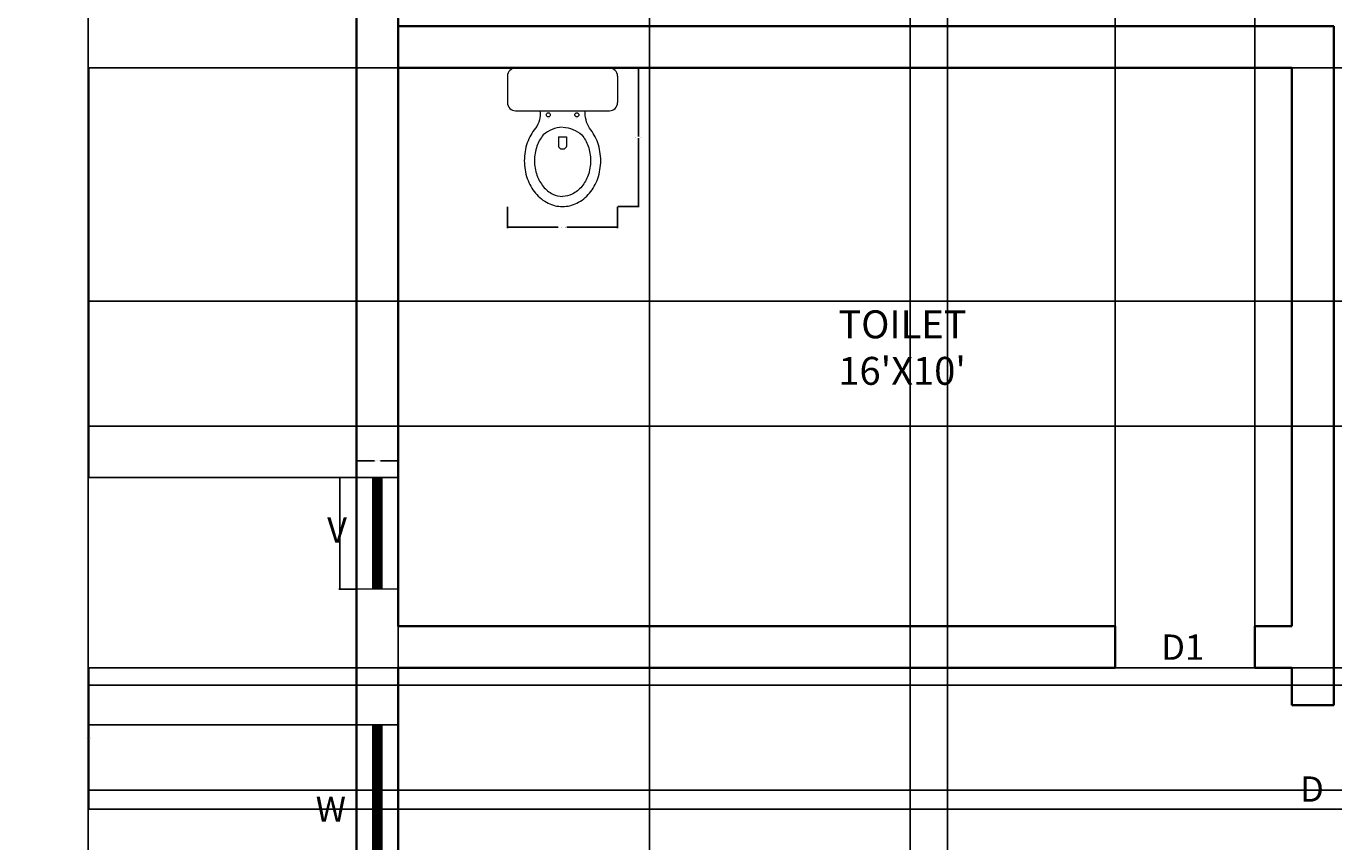
# Model space of a CAD drawing. Units: inches. Extents: x 318 to 927, y -1130 to 13.
# Tile 6 of 17: x 318 to 599, y -867 to -692. Entities that reach past the tile are written whole.
import ezdxf

# ---------------------------------------------------------------- set-up
doc = ezdxf.new("R2010")
doc.units = ezdxf.units.IN
doc.header["$MEASUREMENT"] = 0
for name, color, linetype, lineweight in [('A-ANNO-DIMS', 1, 'Continuous', 18), ('A-ANNO-IDEN', 1, 'Continuous', 13), ('A-AREA-IDEN', 8, 'Continuous', 18), ('A-FLOR-FIXT', 7, 'Continuous', 18), ('A-GLAZ-PATT', 5, 'Continuous', 9), ('wall', 1, 'Continuous', 35), ('win', 5, 'Continuous', 18)]:
    doc.layers.add(name, color=color, linetype=linetype, lineweight=lineweight)
doc.styles.get("Standard").update_dxf_attribs({"font": 'arial.ttf'})
doc.dimstyles.get("Standard").update_dxf_attribs({"dimtxt": 0.18, "dimasz": 0.18, "dimexe": 0.18, "dimexo": 0.0625, "dimgap": 0.09, "dimtad": 0, "dimtih": 1, "dimtoh": 1, "dimdec": 1, "dimzin": 0, "dimdsep": 46, "dimlunit": 4, "dimtxsty": 'Standard', "dimcen": 0.09, "dimadec": 0, "dimazin": 0, "dimtfac": 1, "dimtdec": 1, "dimtofl": 0, "dimtmove": 0, "dimatfit": 3, "dimfxl": 1, "dimtolj": 1, "dimtzin": 0, "dimarcsym": 0})

# ---------------------------------------------------------------- blocks, each defined once
blk = doc.blocks.new('WC-P01')
for p, q in [((-230, 0), (230, 0)), ((-270, -40), (-270, -170)), ((270, -40), (270, -170)), ((-230, -210), (230, -210)), ((-111.4, -210), (-111.4, -210)), ((-20, -337.8), (20, -337.8)), ((-20, -337.8), (-20, -385.7)), ((20, -337.8), (20, -385.7)), ((-18.5, -389.3), (-10.5, -397.3)), ((-10.5, -397.3), (10.5, -397.3)), ((10.5, -397.3), (18.5, -389.3))]:
    blk.add_line(p, q)
for points in [[(-111.4, -210, -0.215497), (-132.6, -295.9, 0.09084), (-172.8, -367.1, 0.083285), (-187.5, -455, 0.083285), (-172.8, -542.9, 0.09084), (-132.6, -614.1, 0.104065), (-70, -663.6, 0.115836), (0, -680, 0.115836), (70, -663.6, 0.104065), (132.6, -614.1, 0.09084), (172.8, -542.9, 0.083285), (187.5, -455, 0.083285)], [(-70, -246.4), (-70, -246.4, 0.104065)], [(70, -246.4), (70, -246.4, 0.115836)], [(187.5, -455, 0.083285), (172.8, -367.1, 0.09084), (132.6, -295.9, -0.156524), (111.4, -210)], [(-1.8, -291.3, 0.171753), (-94.2, -327.9, 0.09084), (-125.5, -383.5, 0.083285), (-137.5, -455, 0.083285), (-125.5, -526.5, 0.09084), (-94.2, -582.1, 0.104065), (-47.7, -618.8, 0.115836), (0, -630, 0.115836)], [(1.8, -291.3, -0.171753), (94.2, -327.9, -0.09084), (125.5, -383.5, -0.083285), (137.5, -455, -0.083285), (125.5, -526.5, -0.09084), (94.2, -582.1, -0.104065), (47.7, -618.8, -0.115836), (0, -630, -0.115836)]]:
    blk.add_lwpolyline(points, format="xyb")
for centre in [(-70, -230), (70, -230)]:
    blk.add_circle(centre, 10)
for centre, radius, start, end in [((-230, -40), 40, 90, 180), ((230, -40), 40, 0, 90), ((-230, -170), 40, 180, 270), ((230, -170), 40, 270, 0), ((-15, -385.7), 5, 180, 225), ((15, -385.7), 5, 315, 0)]:
    blk.add_arc(centre, radius, start, end)
blk = doc.blocks.new('_ArchTick')
at = {"color": 0, "linetype": 'ByBlock', "const_width": 0.15}
blk.add_lwpolyline([(-0.5, -0.5), (0.5, 0.5)], dxfattribs=at)
blk = doc.blocks.new('*D4')
at = {"layer": 'A-ANNO-DIMS', "color": 0, "lineweight": -2, "transparency": 16777216}
blk.add_line((331.26, -82.91), (331.26, -1042.91), dxfattribs=at)
at = {"layer": 'Defpoints', "color": 0, "transparency": 16777216}
for p in [(388.89, -82.91), (331.26, -1042.91), (388.89, -1042.91)]:
    blk.add_point(p, dxfattribs=at)
at = {"layer": 'A-ANNO-DIMS', "color": 0, "lineweight": -2, "transparency": 16777216, "xscale": 6, "yscale": 6, "zscale": 6}
for p, rotation in [((331.26, -82.91), 90), ((331.26, -1042.91), 270)]:
    blk.add_blockref('_ArchTick', p, dxfattribs=dict(at, rotation=rotation))
at = {"layer": 'A-ANNO-DIMS', "color": 0, "transparency": 16777216, "insert": (323.18, -562.91), "char_height": 8, "attachment_point": 5, "rotation": 90}
blk.add_mtext("\\A1;80'", dxfattribs=at)
blk = doc.blocks.new('WIN-36IN')
for p, q in [((0, 36), (9, 36)), ((3.5, 36), (3.5, 0)), ((5.5, 36), (5.5, 0)), ((0, 0), (9, 0))]:
    blk.add_line(p, q)
blk = doc.blocks.new('VENT-24IN')
for p, q in [((9, 24), (0, 24)), ((3.5, 0), (3.5, 24)), ((5.5, 0), (5.5, 24)), ((9, 0), (0, 0))]:
    blk.add_line(p, q)
blk = doc.blocks.new('*D17')
at = {"layer": 'A-ANNO-DIMS', "color": 0, "lineweight": -2, "transparency": 16777216}
for p, q in [((445.06, -700.91), (449.65, -700.91)), ((449.47, -701.09), (449.47, -715.62)), ((449.47, -730.52), (449.47, -715.99)), ((445.06, -730.7), (449.65, -730.7))]:
    blk.add_line(p, q, dxfattribs=at)
at = {"layer": 'A-ANNO-DIMS', "color": 0, "transparency": 16777216}
for points in [[(449.44, -701.09), (449.5, -701.09), (449.47, -700.91)], [(449.44, -730.52), (449.5, -730.52), (449.47, -730.7)]]:
    blk.add_solid(points, dxfattribs=at)
at = {"layer": 'Defpoints', "color": 0, "transparency": 16777216}
for p in [(445, -700.91), (449.47, -700.91), (445, -730.7)]:
    blk.add_point(p, dxfattribs=at)
at = {"layer": 'A-ANNO-DIMS', "color": 0, "transparency": 16777216, "insert": (449.47, -715.81), "char_height": 0.18, "attachment_point": 5}
blk.add_mtext('\\A1;WC 2\'-6" TYP.', dxfattribs=at)
blk = doc.blocks.new('*D18')
at = {"layer": 'A-ANNO-DIMS', "color": 0, "lineweight": -2, "transparency": 16777216}
for p, q in [((421.34, -730.76), (421.34, -735.35)), ((445, -730.76), (445, -735.35)), ((421.52, -735.17), (432.26, -735.17)), ((444.82, -735.17), (434.08, -735.17))]:
    blk.add_line(p, q, dxfattribs=at)
at = {"layer": 'A-ANNO-DIMS', "color": 0, "transparency": 16777216}
for points in [[(421.52, -735.14), (421.52, -735.2), (421.34, -735.17)], [(444.82, -735.14), (444.82, -735.2), (445, -735.17)]]:
    blk.add_solid(points, dxfattribs=at)
at = {"layer": 'Defpoints', "color": 0, "transparency": 16777216}
for p in [(421.34, -730.7), (445, -730.7), (445, -735.17)]:
    blk.add_point(p, dxfattribs=at)
at = {"layer": 'A-ANNO-DIMS', "color": 0, "transparency": 16777216, "insert": (433.17, -735.17), "char_height": 0.18, "attachment_point": 5}
blk.add_mtext('\\A1;1\'-11 1/2" TYP.', dxfattribs=at)
blk = doc.blocks.new('*D21')
at = {"layer": 'A-ANNO-DIMS', "color": 0, "lineweight": -2, "transparency": 16777216}
for p, q in [((388.83, -788.96), (385.11, -788.96)), ((385.29, -789.14), (385.29, -800.78)), ((385.29, -812.78), (385.29, -801.14)), ((388.83, -812.96), (385.11, -812.96))]:
    blk.add_line(p, q, dxfattribs=at)
at = {"layer": 'A-ANNO-DIMS', "color": 0, "transparency": 16777216}
for points in [[(385.26, -789.14), (385.32, -789.14), (385.29, -788.96)], [(385.26, -812.78), (385.32, -812.78), (385.29, -812.96)]]:
    blk.add_solid(points, dxfattribs=at)
at = {"layer": 'Defpoints', "color": 0, "transparency": 16777216}
for p in [(385.29, -788.96), (388.89, -788.96), (388.89, -812.96)]:
    blk.add_point(p, dxfattribs=at)
at = {"layer": 'A-ANNO-DIMS', "color": 0, "transparency": 16777216, "insert": (385.29, -800.96), "char_height": 0.18, "attachment_point": 5}
blk.add_mtext('\\A1;VENT 2\'-0" TYP.', dxfattribs=at)
blk = doc.blocks.new('*D22')
at = {"layer": 'A-ANNO-DIMS', "color": 0, "lineweight": -2, "transparency": 16777216}
for p, q in [((388.89, -788.9), (388.89, -785.18)), ((389.07, -785.36), (392.76, -785.36)), ((397.71, -785.36), (394.03, -785.36)), ((397.89, -788.9), (397.89, -785.18))]:
    blk.add_line(p, q, dxfattribs=at)
at = {"layer": 'A-ANNO-DIMS', "color": 0, "transparency": 16777216}
for points in [[(389.07, -785.33), (389.07, -785.39), (388.89, -785.36)], [(397.71, -785.33), (397.71, -785.39), (397.89, -785.36)]]:
    blk.add_solid(points, dxfattribs=at)
at = {"layer": 'Defpoints', "color": 0, "transparency": 16777216}
for p in [(397.89, -785.36), (388.89, -788.96), (397.89, -788.96)]:
    blk.add_point(p, dxfattribs=at)
at = {"layer": 'A-ANNO-DIMS', "color": 0, "transparency": 16777216, "insert": (393.39, -785.36), "char_height": 0.18, "attachment_point": 5}
blk.add_mtext('\\A1;0\'-9" TYP.', dxfattribs=at)
blk = doc.blocks.new('*D30')
at = {"layer": 'A-ANNO-DIMS', "color": 0, "lineweight": -2, "transparency": 16777216}
for p, q in [((551.89, -820.85), (551.89, -25.23)), ((581.89, -820.85), (581.89, -25.23)), ((552.07, -25.41), (566.56, -25.41)), ((581.71, -25.41), (567.23, -25.41))]:
    blk.add_line(p, q, dxfattribs=at)
at = {"layer": 'A-ANNO-DIMS', "color": 0, "transparency": 16777216}
for points in [[(552.07, -25.38), (552.07, -25.44), (551.89, -25.41)], [(581.71, -25.38), (581.71, -25.44), (581.89, -25.41)]]:
    blk.add_solid(points, dxfattribs=at)
at = {"layer": 'Defpoints', "color": 0, "transparency": 16777216}
for p in [(581.89, -25.41), (551.89, -820.91), (581.89, -820.91)]:
    blk.add_point(p, dxfattribs=at)
at = {"layer": 'A-ANNO-DIMS', "color": 0, "transparency": 16777216, "insert": (566.89, -25.41), "char_height": 0.18, "attachment_point": 5}
blk.add_mtext('\\A1;2\'-6"', dxfattribs=at)
blk = doc.blocks.new('*D35')
at = {"layer": 'A-ANNO-DIMS', "color": 0, "lineweight": -2, "transparency": 16777216}
for p, q in [((397.89, -457.98), (397.89, -1124.59)), ((451.89, -457.98), (451.89, -1124.59)), ((398.07, -1124.41), (424.56, -1124.41)), ((451.71, -1124.41), (425.23, -1124.41))]:
    blk.add_line(p, q, dxfattribs=at)
at = {"layer": 'A-ANNO-DIMS', "color": 0, "transparency": 16777216}
for points in [[(398.07, -1124.38), (398.07, -1124.44), (397.89, -1124.41)], [(451.71, -1124.38), (451.71, -1124.44), (451.89, -1124.41)]]:
    blk.add_solid(points, dxfattribs=at)
at = {"layer": 'Defpoints', "color": 0, "transparency": 16777216}
for p in [(397.89, -457.91), (451.89, -457.91), (451.89, -1124.41)]:
    blk.add_point(p, dxfattribs=at)
at = {"layer": 'A-ANNO-DIMS', "color": 0, "transparency": 16777216, "insert": (424.89, -1124.41), "char_height": 0.18, "attachment_point": 5}
blk.add_mtext('\\A1;4\'-6"', dxfattribs=at)
blk = doc.blocks.new('*D36')
at = {"layer": 'A-ANNO-DIMS', "color": 0, "lineweight": -2, "transparency": 16777216}
for p, q in [((507.89, -457.98), (507.89, -1124.59)), ((515.89, -457.98), (515.89, -1124.59)), ((508.07, -1124.41), (511.57, -1124.41)), ((515.71, -1124.41), (512.22, -1124.41))]:
    blk.add_line(p, q, dxfattribs=at)
at = {"layer": 'A-ANNO-DIMS', "color": 0, "transparency": 16777216}
for points in [[(508.07, -1124.38), (508.07, -1124.44), (507.89, -1124.41)], [(515.71, -1124.38), (515.71, -1124.44), (515.89, -1124.41)]]:
    blk.add_solid(points, dxfattribs=at)
at = {"layer": 'Defpoints', "color": 0, "transparency": 16777216}
for p in [(507.89, -457.91), (515.89, -457.91), (515.89, -1124.41)]:
    blk.add_point(p, dxfattribs=at)
at = {"layer": 'A-ANNO-DIMS', "color": 0, "transparency": 16777216, "insert": (511.89, -1124.41), "char_height": 0.18, "attachment_point": 5}
blk.add_mtext('\\A1;0\'-8"', dxfattribs=at)
blk = doc.blocks.new('*D49')
at = {"layer": 'A-ANNO-DIMS', "color": 0, "lineweight": -2, "transparency": 16777216}
for p, q in [((765.82, -751.08), (331.21, -751.08)), ((331.39, -751.26), (331.39, -764.33)), ((331.39, -777.76), (331.39, -764.69)), ((765.82, -777.94), (331.21, -777.94))]:
    blk.add_line(p, q, dxfattribs=at)
at = {"layer": 'A-ANNO-DIMS', "color": 0, "transparency": 16777216}
for points in [[(331.36, -751.26), (331.42, -751.26), (331.39, -751.08)], [(331.36, -777.76), (331.42, -777.76), (331.39, -777.94)]]:
    blk.add_solid(points, dxfattribs=at)
at = {"layer": 'Defpoints', "color": 0, "transparency": 16777216}
for p in [(765.88, -751.08), (331.39, -777.94), (765.88, -777.94)]:
    blk.add_point(p, dxfattribs=at)
at = {"layer": 'A-ANNO-DIMS', "color": 0, "transparency": 16777216, "insert": (331.39, -764.51), "char_height": 0.18, "attachment_point": 5}
blk.add_mtext('\\A1;2\'-3"', dxfattribs=at)
blk = doc.blocks.new('*D51')
at = {"layer": 'A-ANNO-DIMS', "color": 0, "lineweight": -2, "transparency": 16777216}
for p, q in [((771.33, -700.91), (331.21, -700.91)), ((331.39, -701.09), (331.39, -725.82)), ((331.39, -750.9), (331.39, -726.18)), ((765.82, -751.08), (331.21, -751.08))]:
    blk.add_line(p, q, dxfattribs=at)
at = {"layer": 'A-ANNO-DIMS', "color": 0, "transparency": 16777216}
for points in [[(331.36, -701.09), (331.42, -701.09), (331.39, -700.91)], [(331.36, -750.9), (331.42, -750.9), (331.39, -751.08)]]:
    blk.add_solid(points, dxfattribs=at)
at = {"layer": 'Defpoints', "color": 0, "transparency": 16777216}
for p in [(771.39, -700.91), (331.39, -751.08), (765.88, -751.08)]:
    blk.add_point(p, dxfattribs=at)
at = {"layer": 'A-ANNO-DIMS', "color": 0, "transparency": 16777216, "insert": (331.39, -726), "char_height": 0.18, "attachment_point": 5}
blk.add_mtext('\\A1;4\'-2"', dxfattribs=at)
blk = doc.blocks.new('*D52')
at = {"layer": 'A-ANNO-DIMS', "color": 0, "lineweight": -2, "transparency": 16777216}
for p, q in [((829.83, -829.91), (331.21, -829.91)), ((331.39, -830.09), (331.39, -844.92)), ((331.39, -860.11), (331.39, -845.29)), ((829.83, -860.29), (331.21, -860.29))]:
    blk.add_line(p, q, dxfattribs=at)
at = {"layer": 'A-ANNO-DIMS', "color": 0, "transparency": 16777216}
for points in [[(331.36, -830.09), (331.42, -830.09), (331.39, -829.91)], [(331.36, -860.11), (331.42, -860.11), (331.39, -860.29)]]:
    blk.add_solid(points, dxfattribs=at)
at = {"layer": 'Defpoints', "color": 0, "transparency": 16777216}
for p in [(829.89, -829.91), (331.39, -860.29), (829.89, -860.29)]:
    blk.add_point(p, dxfattribs=at)
at = {"layer": 'A-ANNO-DIMS', "color": 0, "transparency": 16777216, "insert": (331.39, -845.1), "char_height": 0.18, "attachment_point": 5}
blk.add_mtext('\\A1;2\'-6 1/2"', dxfattribs=at)
blk = doc.blocks.new('*D54')
at = {"layer": 'A-ANNO-DIMS', "color": 0, "lineweight": -2, "transparency": 16777216}
for p, q in [((842.8, -833.64), (331.21, -833.64)), ((331.39, -833.82), (331.39, -844.73)), ((331.39, -856), (331.39, -845.09)), ((843.25, -856.18), (331.21, -856.18))]:
    blk.add_line(p, q, dxfattribs=at)
at = {"layer": 'A-ANNO-DIMS', "color": 0, "transparency": 16777216}
for points in [[(331.36, -833.82), (331.42, -833.82), (331.39, -833.64)], [(331.36, -856), (331.42, -856), (331.39, -856.18)]]:
    blk.add_solid(points, dxfattribs=at)
at = {"layer": 'Defpoints', "color": 0, "transparency": 16777216}
for p in [(842.87, -833.64), (331.39, -856.18), (843.31, -856.18)]:
    blk.add_point(p, dxfattribs=at)
at = {"layer": 'A-ANNO-DIMS', "color": 0, "transparency": 16777216, "insert": (331.39, -844.91), "char_height": 0.18, "attachment_point": 5}
blk.add_mtext('\\A1;1\'-10 1/2"', dxfattribs=at)
blk = doc.blocks.new('*D69')
at = {"layer": 'A-ANNO-DIMS', "color": 0, "lineweight": -2, "transparency": 16777216}
for p, q in [((397.83, -700.91), (331.21, -700.91)), ((331.39, -701.09), (331.39, -744.76)), ((331.39, -788.78), (331.39, -745.12)), ((397.83, -788.96), (331.21, -788.96))]:
    blk.add_line(p, q, dxfattribs=at)
at = {"layer": 'A-ANNO-DIMS', "color": 0, "transparency": 16777216}
for points in [[(331.36, -701.09), (331.42, -701.09), (331.39, -700.91)], [(331.36, -788.78), (331.42, -788.78), (331.39, -788.96)]]:
    blk.add_solid(points, dxfattribs=at)
at = {"layer": 'Defpoints', "color": 0, "transparency": 16777216}
for p in [(397.89, -700.91), (331.39, -788.96), (397.89, -788.96)]:
    blk.add_point(p, dxfattribs=at)
at = {"layer": 'A-ANNO-DIMS', "color": 0, "transparency": 16777216, "insert": (331.39, -744.94), "char_height": 0.18, "attachment_point": 5}
blk.add_mtext('\\A1;7\'-4"', dxfattribs=at)
blk = doc.blocks.new('*D70')
at = {"layer": 'A-ANNO-DIMS', "color": 0, "lineweight": -2, "transparency": 16777216}
for p, q in [((397.83, -829.91), (331.21, -829.91)), ((331.39, -830.09), (331.39, -835.85)), ((331.39, -841.97), (331.39, -836.21)), ((397.83, -842.15), (331.21, -842.15))]:
    blk.add_line(p, q, dxfattribs=at)
at = {"layer": 'A-ANNO-DIMS', "color": 0, "transparency": 16777216}
for points in [[(331.36, -830.09), (331.42, -830.09), (331.39, -829.91)], [(331.36, -841.97), (331.42, -841.97), (331.39, -842.15)]]:
    blk.add_solid(points, dxfattribs=at)
at = {"layer": 'Defpoints', "color": 0, "transparency": 16777216}
for p in [(397.89, -829.91), (331.39, -842.15), (397.89, -842.15)]:
    blk.add_point(p, dxfattribs=at)
at = {"layer": 'A-ANNO-DIMS', "color": 0, "transparency": 16777216, "insert": (331.39, -836.03), "char_height": 0.18, "attachment_point": 5}
blk.add_mtext('\\A1;1\'-0"', dxfattribs=at)

msp = doc.modelspace()

# ---------------------------------------------------------------- hatches: boundary and pattern name
at = {"layer": 'A-GLAZ-PATT'}
h = msp.add_hatch(dxfattribs=at)
h.set_pattern_fill('ANSI31', color=256)
h.paths.add_polyline_path([(787.43, -1037.41), (751.43, -1037.41), (751.43, -1039.41), (787.43, -1039.41)])
h.paths.add_polyline_path([(583.67, -1037.41), (547.67, -1037.41), (547.67, -1039.41), (583.67, -1039.41)])
h.paths.add_polyline_path([(394.39, -842.15), (392.39, -842.15), (392.39, -878.15), (394.39, -878.15)])
h.paths.add_polyline_path([(394.39, -788.96), (392.39, -788.96), (392.39, -812.96), (394.39, -812.96)])

# ---------------------------------------------------------------- linework, layer by layer
at = {"layer": 'wall'}
for p, q in [((388.89, -82.91), (388.89, -1042.91)), ((397.89, -547.91), (397.89, -820.91)), ((397.89, -691.91), (598.89, -691.91)), ((598.89, -691.91), (598.89, -837.91)), ((397.89, -700.91), (589.89, -700.91)), ((589.89, -700.91), (589.89, -820.91)), ((397.89, -820.91), (551.89, -820.91)), ((551.89, -820.91), (551.89, -829.91)), ((581.89, -820.91), (581.89, -829.91)), ((581.89, -820.91), (589.89, -820.91)), ((397.89, -829.91), (551.89, -829.91)), ((397.89, -829.91), (397.89, -1033.91)), ((581.89, -829.91), (589.89, -829.91)), ((589.89, -829.91), (589.89, -837.91)), ((589.89, -837.91), (598.89, -837.91))]:
    msp.add_line(p, q, dxfattribs=at)

# ---------------------------------------------------------------- block references
at = {"layer": 'A-FLOR-FIXT', "xscale": 0.0438047028060103, "yscale": 0.0438047028060103, "zscale": 0.0438047028060103}
msp.add_blockref('WC-P01', (433.17, -700.91), dxfattribs=at)
at = {"layer": 'win'}
msp.add_blockref('VENT-24IN', (388.89, -812.96), dxfattribs=at)
at = {"layer": 'win', "rotation": 180}
msp.add_blockref('WIN-36IN', (397.89, -842.15), dxfattribs=at)

# ---------------------------------------------------------------- texts
at = {"layer": 'A-ANNO-IDEN'}
for s, height, p in [('V', 5.44, (382.59, -802.94)), ('D1', 5.444, (561.8, -828.16)), ('D', 5.44, (591.65, -858.67)), ('W', 5.44, (380.13, -862.99))]:
    msp.add_text(s, height=height, dxfattribs=at).set_placement(p)
at = {"layer": 'A-AREA-IDEN', "insert": (479.6, -753.03), "char_height": 6, "attachment_point": 1}
msp.add_mtext_dynamic_manual_height_columns("       TOILET\\P       16'X10'", width=54.3765, gutter_width=1, heights=[0], dxfattribs=at)

# ---------------------------------------------------------------- dimensions: what is measured, and where the dimension line sits
at = {"layer": 'A-ANNO-DIMS'}
for base, p1, p2, picture, middle in [((581.89, -25.41), (551.89, -820.91), (581.89, -820.91), '*D30', (566.89, -25.41)), ((451.89, -1124.41), (397.89, -457.91), (451.89, -457.91), '*D35', (424.89, -1124.41)), ((515.89, -1124.41), (507.89, -457.91), (515.89, -457.91), '*D36', (511.89, -1124.41))]:
    dim = msp.add_linear_dim(base=base, p1=p1, p2=p2, dimstyle='Standard', override={"dimdec": 1, "dimlfac": 1, "dimrnd": 0, "dimzin": 1, "dimdsep": 46, "dimlunit": 4, "dimfrac": 2}, dxfattribs=at)
    dim.commit()
    dim.dimension.update_dxf_attribs({"geometry": picture, "text_midpoint": middle})
for base, p1, p2, override, picture, middle in [((331.26, -1042.91), (388.89, -82.91), (388.89, -1042.91), {"dimtxt": 8, "dimasz": 6, "dimgap": 4, "dimtad": 1, "dimtih": 0, "dimblk1": 'ArchTick', "dimblk2": 'ArchTick', "dimsah": 1, "dimse1": 1, "dimse2": 1, "dimclrd": 0, "dimclre": 0, "dimclrt": 0}, '*D4', (323.18, -562.91)), ((331.39, -751.08), (771.39, -700.91), (765.88, -751.08), {"dimdec": 1, "dimlfac": 1, "dimrnd": 0, "dimzin": 1, "dimdsep": 46, "dimlunit": 4, "dimfrac": 2}, '*D51', (331.39, -726)), ((331.3942, -788.9613), (397.8942, -700.9129), (397.8942, -788.9613), {"dimdec": 1, "dimlfac": 1, "dimrnd": 0, "dimzin": 1, "dimdsep": 46, "dimlunit": 4, "dimfrac": 2}, '*D69', (331.3942, -744.9371)), ((331.39, -777.94), (765.88, -751.08), (765.88, -777.94), {"dimdec": 1, "dimlfac": 1, "dimrnd": 0, "dimzin": 1, "dimdsep": 46, "dimlunit": 4, "dimfrac": 2}, '*D49', (331.39, -764.51)), ((331.39, -860.29), (829.89, -829.91), (829.89, -860.29), {"dimdec": 1, "dimlfac": 1, "dimrnd": 0, "dimzin": 1, "dimdsep": 46, "dimlunit": 4, "dimfrac": 2}, '*D52', (331.39, -845.1)), ((331.39, -842.15), (397.89, -829.91), (397.89, -842.15), {"dimdec": 1, "dimlfac": 1, "dimrnd": 0, "dimzin": 1, "dimdsep": 46, "dimlunit": 4, "dimfrac": 2}, '*D70', (331.39, -836.03)), ((331.39, -856.18), (842.87, -833.64), (843.31, -856.18), {"dimdec": 1, "dimlfac": 1, "dimrnd": 0, "dimzin": 1, "dimdsep": 46, "dimlunit": 4, "dimfrac": 2}, '*D54', (331.39, -844.91))]:
    dim = msp.add_linear_dim(base=base, p1=p1, p2=p2, angle=90, dimstyle='Standard', override=override, dxfattribs=at)
    dim.commit()
    dim.dimension.update_dxf_attribs({"geometry": picture, "text_midpoint": middle})
for base, p1, p2, text, picture, middle in [((449.47, -700.91), (445, -730.7), (445, -700.91), 'WC <> TYP.', '*D17', (449.47, -715.81)), ((385.29, -788.96), (388.89, -812.96), (388.89, -788.96), 'VENT <> TYP.', '*D21', (385.29, -800.96))]:
    dim = msp.add_linear_dim(base=base, p1=p1, p2=p2, angle=90, text=text, dimstyle='Standard', override={"dimdec": 1, "dimlfac": 1, "dimrnd": 0, "dimzin": 1, "dimdsep": 46, "dimlunit": 4, "dimfrac": 2}, dxfattribs=at)
    dim.commit()
    dim.dimension.update_dxf_attribs({"geometry": picture, "text_midpoint": middle})
for base, p1, p2, picture, middle in [((445, -735.17), (421.34, -730.7), (445, -730.7), '*D18', (433.17, -735.17)), ((397.89, -785.36), (388.89, -788.96), (397.89, -788.96), '*D22', (393.39, -785.36))]:
    dim = msp.add_linear_dim(base=base, p1=p1, p2=p2, text='<> TYP.', dimstyle='Standard', override={"dimdec": 1, "dimlfac": 1, "dimrnd": 0, "dimzin": 1, "dimdsep": 46, "dimlunit": 4, "dimfrac": 2}, dxfattribs=at)
    dim.commit()
    dim.dimension.update_dxf_attribs({"geometry": picture, "text_midpoint": middle})

doc.saveas('drawing.dxf')
